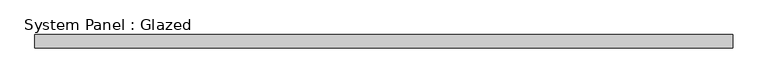
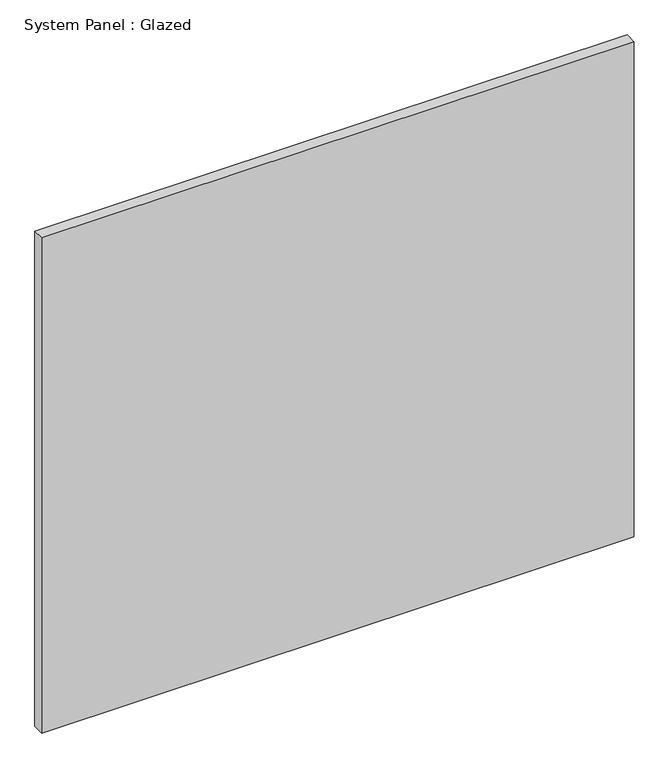
"""IFC4 building model written with IfcOpenShell, lengths in millimetres: plate geometry, System Panel : Glazed."""

from ifc_helpers import new_model, si_unit, origin, origin_with_axes, place, context, project, spatial, polyline, outline, extrude, source, transform, mapped, element, save


def system_panel_glazed_fdf8efc7(model_context):
    return source(origin(), model_context, "Body", "SweptSolid", [
        extrude(outline(polyline([(654.05, 19.05), (-654.05, 19.05), (-654.05, 44.45), (654.05, 44.45), (654.05, 19.05)])), origin_with_axes(), (0.0, 0.0, 1.0), 1155.7),
    ])


if __name__ == "__main__":
    model = new_model("IFC4")
    model_context = context("Model", 3, world=origin())
    ifc_project = project(units=[si_unit("LENGTHUNIT", "METRE", prefix="MILLI")], contexts=[model_context])
    site = spatial("IfcSite", under=ifc_project)
    building = spatial("IfcBuilding", under=site)
    placement = place(None, origin())
    system_panel_glazed_shape = system_panel_glazed_fdf8efc7(model_context)
    element("IfcPlate", 1, ObjectType="System Panel : Glazed", at=placement, inside=building, context=model_context, shape_type="MappedRepresentation", body=[
        mapped(system_panel_glazed_shape, transform((0.0, 0.0, 0.0), x_axis=(1.0, 0.0, 0.0), y_axis=(0.0, 1.0, 0.0), z_axis=(0.0, 0.0, 1.0))),
    ])
    save(model, "model.ifc")

# Revit data of these elements
# Type "System Panel : Glazed"
#   Construction Type Id = "GSP4R"
#   Analytic Construction = "1/8 in Pilkington single glazing"
#   Visual Light Transmittance = 0.9
#   Solar Heat Gain Coefficient = 0.86
#   Heat Transfer Coefficient (U) = 1.18115 BTU/(h·ft²·°F)
# Element 1 (IfcPlate, "System Panel : Glazed")
#   Materials on its faces: "Glass"
# Materials
#   "Glass": class "Glass", colour RGB 0 128 192, transparency 0.75, Description = "Soda Lime Glass", Cost = 0
